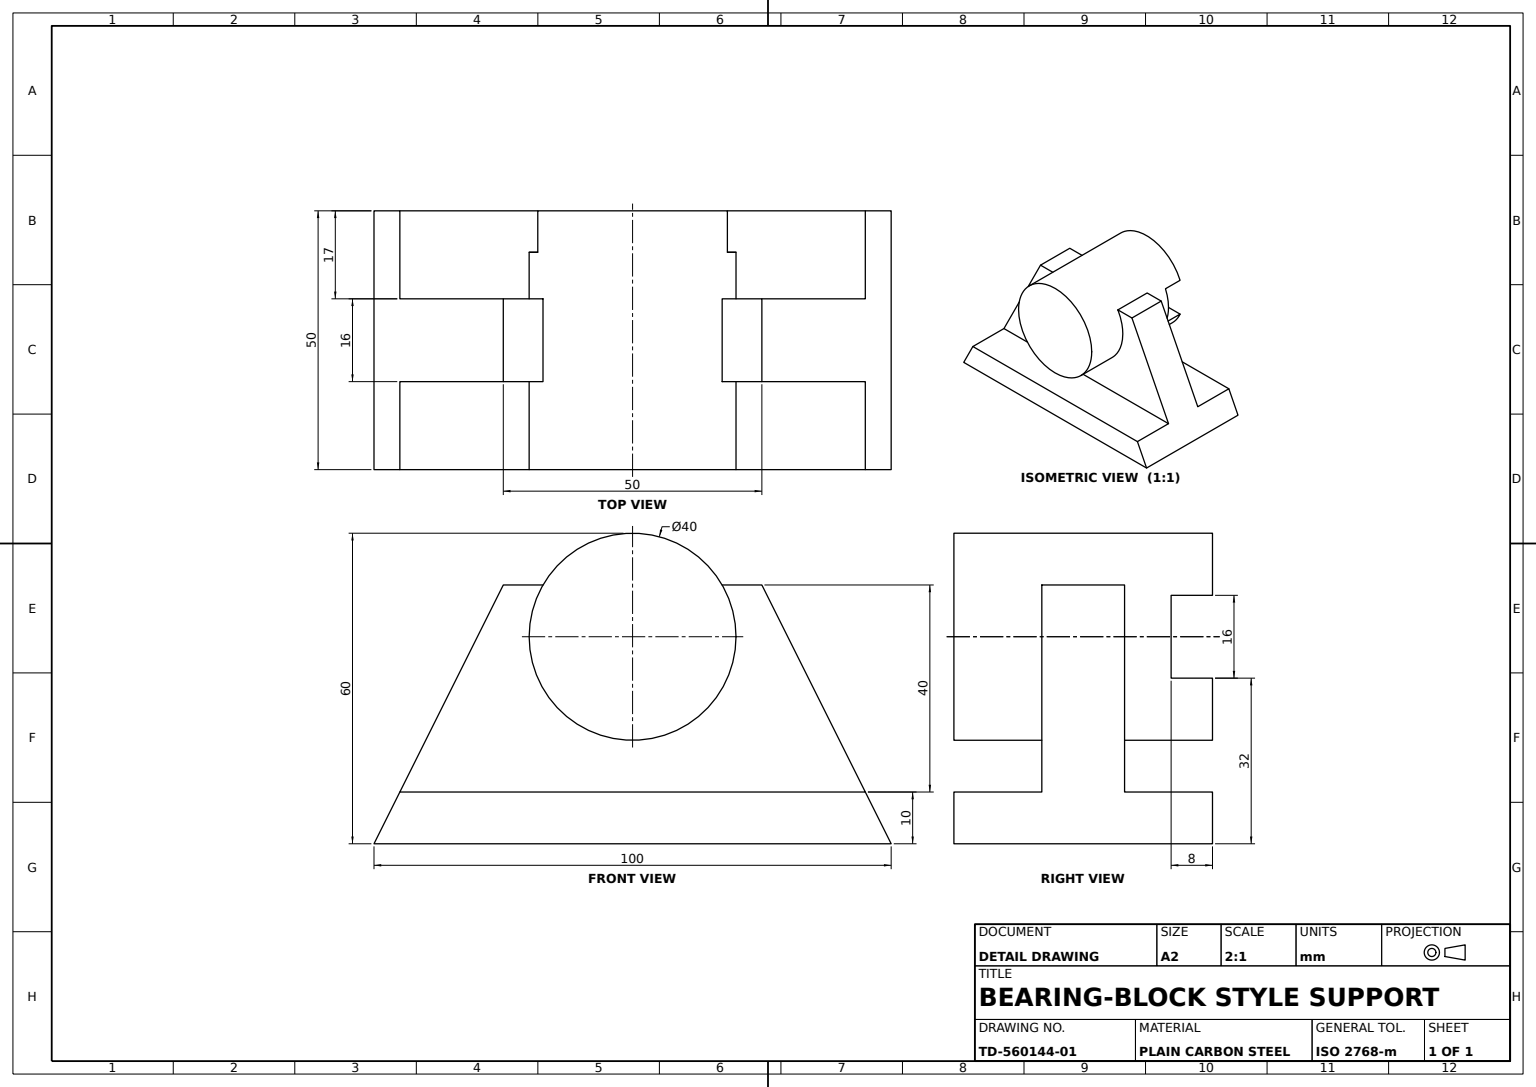
SolidWorks part; units mm, degrees
material "Plain Carbon Steel"
ref_plane "Front Plane" through (0, 0, 0) normal (0, 0, 1) x (1, 0, 0)
ref_plane "Top Plane" through (0, 0, 0) normal (0, 1, 0) x (1, 0, 0)
ref_plane "Right Plane" through (0, 0, 0) normal (1, 0, 0) x (0, 0, -1)
sketch "Base Plate Sketch" plane through (0, 0, 0) normal (0, 0, 1) x (1, 0, 0)
  line L0 (0, 0) -> (109.9678, 0) construction
  line L1 (0, 0) -> (100, 0)
  line L2 (100, 0) -> (95, 10)
  line L3 (95, 10) -> (5, 10)
  line L4 (5, 10) -> (0, 0)
  dimension "D1" = 100
  dimension "D2" = 90
  dimension "D3" = 5
  dimension "D4" = 10
extrude "Base Plate" add sketch "Base Plate Sketch" along normal mid plane 50
sketch "Support Upright Sketch" plane through (0, 0, 0) normal (0, 0, 1) x (1, 0, 0)
  line L0 (5, 10) -> (95, 10)
  line L1 (95, 10) -> (75, 50)
  line L2 (75, 50) -> (25, 50)
  line L3 (25, 50) -> (5, 10)
  line L4 (50, 10) -> (50, 38.828) construction
  dimension "D1" = 25
  dimension "D2" = 25
  dimension "D3" = 40
extrude "Support Upright" add sketch "Support Upright Sketch" along normal mid plane 16
sketch "Shaft Cylinder Sketch" plane through (0, 0, 0) normal (0, 0, 1) x (1, 0, 0)
  line L0 (75, 50) -> (25, 50) construction
  line L1 (50, 10) -> (50, 63.2617) construction
  line L2 (5, 10) -> (95, 10) construction
  circle A0 centre (50, 40) radius 20
  dimension "D2" = 40
  dimension "D1" = 10
extrude "Shaft Cylinder Ø40" add sketch "Shaft Cylinder Sketch" along normal mid plane 50
sketch "Shaft End Notch Sketch" plane through (0, 0, -25) normal (0, 0, -1) x (-1, 0, 0)
  line L0 (-31.6697, 48) -> (-68.3303, 48)
  line L2 (-31.6697, 32) -> (-68.3303, 32)
  circle A0 centre (-50, 40) radius 20 construction
  arc A1 (-31.6697, 32) -> (-31.6697, 48) centre (-50, 40) ccw
  arc A2 (-68.3303, 48) -> (-68.3303, 32) centre (-50, 40) ccw
  point P0 (-14.2015, 48)
  point P1 (-14.2015, 40)
  point P3 (-83.9922, 48)
  point P4 (-83.9922, 40)
  point P5 (-14.2015, 32)
  point P6 (-83.9922, 32)
  dimension "D1" = 18.3303
extrude "Shaft End Notch" cut sketch "Shaft End Notch Sketch" against normal blind 8
